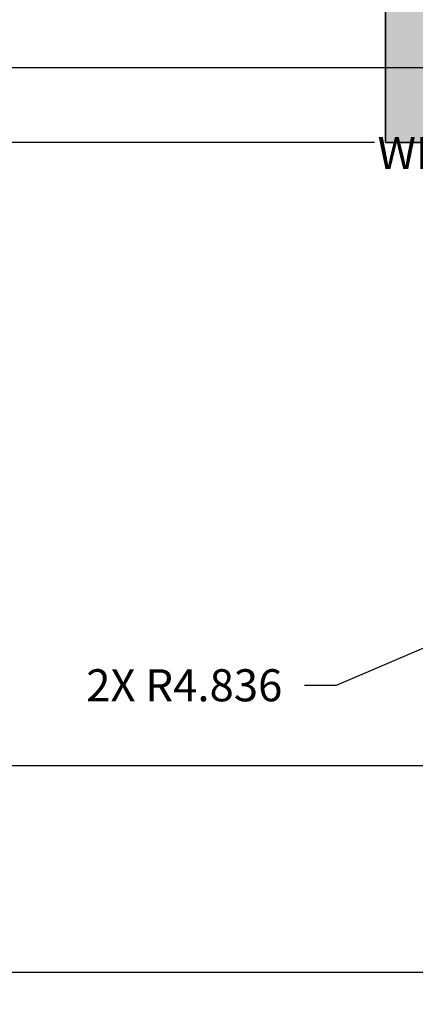
# Model space of a CAD drawing. Units: metres. Extents: x 4298.5 to 4325.2, y 2075 to 2095.8.
# Tile 2 of 35: x 4303.6 to 4305.8, y 2075 to 2080.5. Entities that reach past the tile are written whole.
import ezdxf

# ---------------------------------------------------------------- set-up
doc = ezdxf.new("R2010")
doc.units = ezdxf.units.M
for name, color, linetype, lineweight in [('A-ANNO-DIMS', 2, 'Continuous', 18), ('A-WALL', 7, 'Continuous', 35), ('A-WALL-PATT', 252, 'Continuous', 13)]:
    doc.layers.add(name, color=color, linetype=linetype, lineweight=lineweight)
doc.styles.get("Standard").update_dxf_attribs({"font": 'arial.ttf'})
doc.dimstyles.get("Standard").update_dxf_attribs({"dimtxt": 0.18, "dimasz": 0.18, "dimexe": 0.18, "dimexo": 0.0625, "dimgap": 0.09, "dimtad": 0, "dimtih": 1, "dimtoh": 1, "dimdec": 4, "dimzin": 0, "dimdsep": 46, "dimtxsty": 'Standard', "dimcen": 0.09, "dimadec": 0, "dimazin": 0, "dimtfac": 1, "dimtdec": 4, "dimtofl": 0, "dimtmove": 0, "dimatfit": 3, "dimfxl": 1, "dimtolj": 1, "dimtzin": 0, "dimarcsym": 0})

# ---------------------------------------------------------------- blocks, each defined once
blk = doc.blocks.new('*D23')
at = {"layer": 'A-ANNO-DIMS', "color": 0, "lineweight": -2, "transparency": 16777216}
for p, q in [((4308.1606, 2079.8556), (4308.1606, 2079.5881)), ((4309.1606, 2079.8556), (4309.1606, 2079.5881)), ((4308.1606, 2079.7681), (4307.9806, 2079.7681)), ((4308.9806, 2079.7681), (4308.3406, 2079.7681))]:
    blk.add_line(p, q, dxfattribs=at)
at = {"layer": 'A-ANNO-DIMS', "color": 0, "transparency": 16777216}
for points in [[(4308.3406, 2079.7981), (4308.3406, 2079.7381), (4308.1606, 2079.7681)], [(4308.9806, 2079.7981), (4308.9806, 2079.7381), (4309.1606, 2079.7681)]]:
    blk.add_solid(points, dxfattribs=at)
at = {"layer": 'Defpoints', "color": 0, "transparency": 16777216}
for p in [(4308.1606, 2079.9181), (4309.1606, 2079.9181), (4308.1606, 2079.7681)]:
    blk.add_point(p, dxfattribs=at)
at = {"layer": 'A-ANNO-DIMS', "color": 0, "transparency": 16777216, "insert": (4306.7086, 2079.7681), "char_height": 0.18, "attachment_point": 5}
blk.add_mtext('\\A1;WINDOW W1 1 TYP.', dxfattribs=at)
blk = doc.blocks.new('*D47')
at = {"layer": 'A-ANNO-DIMS', "color": 0, "lineweight": -2, "transparency": 16777216}
for p, q in [((4300.4306, 2084.4956), (4300.4306, 2074.9896)), ((4322.8106, 2084.4956), (4322.8106, 2074.9896)), ((4300.6106, 2075.1696), (4311.2252, 2075.1696)), ((4322.6306, 2075.1696), (4312.016, 2075.1696))]:
    blk.add_line(p, q, dxfattribs=at)
at = {"layer": 'A-ANNO-DIMS', "color": 0, "transparency": 16777216}
for points in [[(4300.6106, 2075.1996), (4300.6106, 2075.1396), (4300.4306, 2075.1696)], [(4322.6306, 2075.1996), (4322.6306, 2075.1396), (4322.8106, 2075.1696)]]:
    blk.add_solid(points, dxfattribs=at)
at = {"layer": 'Defpoints', "color": 0, "transparency": 16777216}
for p in [(4300.4306, 2084.5581), (4322.8106, 2084.5581), (4322.8106, 2075.1696)]:
    blk.add_point(p, dxfattribs=at)
at = {"layer": 'A-ANNO-DIMS', "color": 0, "transparency": 16777216, "insert": (4311.6206, 2075.1696), "char_height": 0.18, "attachment_point": 5}
blk.add_mtext('\\A1;22.38', dxfattribs=at)
blk = doc.blocks.new('*D51')
at = {"layer": 'A-ANNO-DIMS', "color": 0, "lineweight": -2, "transparency": 16777216}
for p, q in [((4305.5981, 2084.5581), (4299.0921, 2084.5581)), ((4299.2721, 2084.3781), (4299.2721, 2082.375)), ((4299.2721, 2080.0081), (4299.2721, 2082.0111)), ((4305.5981, 2079.8281), (4299.0921, 2079.8281))]:
    blk.add_line(p, q, dxfattribs=at)
at = {"layer": 'A-ANNO-DIMS', "color": 0, "transparency": 16777216}
for points in [[(4299.2421, 2084.3781), (4299.3021, 2084.3781), (4299.2721, 2084.5581)], [(4299.2421, 2080.0081), (4299.3021, 2080.0081), (4299.2721, 2079.8281)]]:
    blk.add_solid(points, dxfattribs=at)
at = {"layer": 'Defpoints', "color": 0, "transparency": 16777216}
for p in [(4305.6606, 2084.5581), (4299.2721, 2079.8281), (4305.6606, 2079.8281)]:
    blk.add_point(p, dxfattribs=at)
at = {"layer": 'A-ANNO-DIMS', "color": 0, "transparency": 16777216, "insert": (4299.2721, 2082.1931), "char_height": 0.18, "attachment_point": 5}
blk.add_mtext('\\A1;4.73', dxfattribs=at)
blk = doc.blocks.new('*D54')
at = {"layer": 'A-ANNO-DIMS', "color": 0, "lineweight": -2, "transparency": 16777216}
for p, q in [((4305.5981, 2079.8281), (4299.0921, 2079.8281)), ((4299.2721, 2079.6481), (4299.2721, 2078.26)), ((4299.2721, 2076.5081), (4299.2721, 2077.8961)), ((4309.0981, 2076.3281), (4299.0921, 2076.3281))]:
    blk.add_line(p, q, dxfattribs=at)
at = {"layer": 'A-ANNO-DIMS', "color": 0, "transparency": 16777216}
for points in [[(4299.2421, 2079.6481), (4299.3021, 2079.6481), (4299.2721, 2079.8281)], [(4299.2421, 2076.5081), (4299.3021, 2076.5081), (4299.2721, 2076.3281)]]:
    blk.add_solid(points, dxfattribs=at)
at = {"layer": 'Defpoints', "color": 0, "transparency": 16777216}
for p in [(4305.6606, 2079.8281), (4299.2721, 2076.3281), (4309.1606, 2076.3281)]:
    blk.add_point(p, dxfattribs=at)
at = {"layer": 'A-ANNO-DIMS', "color": 0, "transparency": 16777216, "insert": (4299.2721, 2078.0781), "char_height": 0.18, "attachment_point": 5}
blk.add_mtext('\\A1;3.5', dxfattribs=at)
blk = doc.blocks.new('*D64')
at = {"layer": 'A-ANNO-DIMS', "color": 0, "lineweight": -2, "transparency": 16777216}
for p, q in [((4312.1097, 2081.1221), (4299.0921, 2081.1221)), ((4299.2721, 2080.9421), (4299.2721, 2080.427)), ((4312.1097, 2080.247), (4299.0921, 2080.247)), ((4299.2721, 2080.247), (4299.2721, 2080.067)), ((4299.2721, 2080.067), (4299.0921, 2080.067))]:
    blk.add_line(p, q, dxfattribs=at)
at = {"layer": 'A-ANNO-DIMS', "color": 0, "transparency": 16777216}
for points in [[(4299.2421, 2080.9421), (4299.3021, 2080.9421), (4299.2721, 2081.1221)], [(4299.2421, 2080.427), (4299.3021, 2080.427), (4299.2721, 2080.247)]]:
    blk.add_solid(points, dxfattribs=at)
at = {"layer": 'Defpoints', "color": 0, "transparency": 16777216}
for p in [(4312.1722, 2081.1221), (4299.2721, 2080.247), (4312.1722, 2080.247)]:
    blk.add_point(p, dxfattribs=at)
at = {"layer": 'A-ANNO-DIMS', "color": 0, "transparency": 16777216, "insert": (4298.7681, 2080.067), "char_height": 0.18, "attachment_point": 5}
blk.add_mtext('\\A1;0.88', dxfattribs=at)
blk = doc.blocks.new('*D78')
at = {"layer": 'A-ANNO-DIMS', "color": 0, "lineweight": -2, "transparency": 16777216}
for p, q in [((4312.4969, 2079.7393), (4312.4969, 2079.9193)), ((4312.4069, 2079.8293), (4312.5869, 2079.8293)), ((4305.3847, 2076.7806), (4307.8863, 2077.853)), ((4305.2047, 2076.7806), (4305.3847, 2076.7806))]:
    blk.add_line(p, q, dxfattribs=at)
at = {"layer": 'A-ANNO-DIMS', "color": 0, "transparency": 16777216}
blk.add_solid([(4307.8745, 2077.8806), (4307.8981, 2077.8254), (4308.0518, 2077.9239)], dxfattribs=at)
at = {"layer": 'Defpoints', "color": 0, "transparency": 16777216}
for p in [(4312.4969, 2079.8293), (4308.0518, 2077.9239)]:
    blk.add_point(p, dxfattribs=at)
at = {"layer": 'A-ANNO-DIMS', "color": 0, "transparency": 16777216, "insert": (4304.53, 2076.7806), "char_height": 0.18, "attachment_point": 5}
blk.add_mtext('\\A1;2X R4.836', dxfattribs=at)

msp = doc.modelspace()

# ---------------------------------------------------------------- hatches: boundary and pattern name
at = {"layer": 'A-WALL-PATT'}
h = msp.add_hatch(color=256, dxfattribs=at)
h.dxf.hatch_style = 1
h.paths.add_polyline_path([(4308.7606, 2094.4781), (4308.1606, 2094.4781), (4307.4606, 2094.4781), (4307.4606, 2094.2481), (4308.2706, 2094.2481), (4308.2706, 2094.1281), (4308.3906, 2094.1281), (4308.3906, 2094.2481), (4308.7606, 2094.2481)])
h.paths.add_polyline_path([(4310.1206, 2094.4781), (4309.5206, 2094.4781), (4309.5206, 2094.2481), (4309.8906, 2094.2481), (4309.8906, 2092.2481), (4308.3906, 2092.2481), (4308.3906, 2093.4281), (4308.2706, 2093.4281), (4308.2706, 2092.0181), (4309.8906, 2092.0181), (4309.8906, 2087.0181), (4309.7706, 2087.0181), (4309.7706, 2086.7881), (4309.8906, 2086.7881), (4311.9406, 2086.7881), (4311.9406, 2087.0181), (4310.1206, 2087.0181), (4310.1206, 2089.0181), (4310.2406, 2089.0181), (4310.2406, 2089.1381), (4310.1206, 2089.1381), (4310.1206, 2092.0181), (4310.3078, 2092.0181), (4310.3078, 2092.2481), (4310.1206, 2092.2481)])
h.paths.add_polyline_path([(4311.7406, 2092.2481), (4311.0678, 2092.2481), (4311.0678, 2092.0181), (4311.7406, 2092.0181)], flags=17)
h.paths.add_polyline_path([(4313.1733, 2092.2481), (4312.5006, 2092.2481), (4312.5006, 2092.0181), (4313.1733, 2092.0181)])
h.paths.add_polyline_path([(4314.5378, 2092.2481), (4314.1206, 2092.2481), (4313.9333, 2092.2481), (4313.9333, 2092.0181), (4314.1206, 2092.0181), (4314.1206, 2087.0181), (4314.0006, 2087.0181), (4314.0006, 2086.7881), (4314.1206, 2086.7881), (4315.5718, 2086.7881), (4315.5718, 2087.0181), (4314.3506, 2087.0181), (4314.3506, 2092.0181), (4314.5378, 2092.0181)])
h.paths.add_polyline_path([(4315.9706, 2092.2481), (4315.2978, 2092.2481), (4315.2978, 2092.0181), (4315.9706, 2092.0181)])
h.paths.add_polyline_path([(4317.4033, 2092.2481), (4316.7306, 2092.2481), (4316.7306, 2092.0181), (4317.4033, 2092.0181)])
h.paths.add_polyline_path([(4318.9506, 2092.2481), (4318.3506, 2092.2481), (4318.1633, 2092.2481), (4318.1633, 2092.0181), (4318.3506, 2092.0181), (4318.3506, 2091.8981), (4318.5806, 2091.8981), (4318.5806, 2092.0181), (4318.9506, 2092.0181)])
h.paths.add_polyline_path([(4321.0106, 2092.2481), (4319.7106, 2092.2481), (4319.7106, 2092.0181), (4320.0806, 2092.0181), (4320.0806, 2090.0181), (4318.5806, 2090.0181), (4318.5806, 2091.1981), (4318.3506, 2091.1981), (4318.3506, 2090.0181), (4318.3506, 2087.0181), (4318.2306, 2087.0181), (4318.2306, 2086.7881), (4318.3506, 2086.7881), (4318.3506, 2086.3081), (4318.5806, 2086.3081), (4318.5806, 2089.7881), (4321.7806, 2089.7881), (4321.7806, 2090.0181), (4320.2006, 2090.0181), (4320.2006, 2092.0181), (4321.0106, 2092.0181)])
h.paths.add_polyline_path([(4322.8106, 2092.2481), (4321.7706, 2092.2481), (4321.7706, 2092.0181), (4322.5806, 2092.0181), (4322.5806, 2091.2831), (4322.8106, 2091.2831)])
h.paths.add_polyline_path([(4322.8106, 2090.5231), (4322.5806, 2090.5231), (4322.5806, 2089.7881), (4322.5806, 2089.5254), (4322.8106, 2089.5254), (4322.8106, 2090.0181)])
h.paths.add_polyline_path([(4322.8106, 2088.7654), (4322.5806, 2088.7654), (4322.5806, 2087.6681), (4322.8106, 2087.6681)])
h.paths.add_polyline_path([(4322.8106, 2086.9081), (4322.5806, 2086.9081), (4322.5806, 2085.8107), (4322.8106, 2085.8107)])
h.paths.add_polyline_path([(4322.8106, 2085.0507), (4322.5806, 2085.0507), (4322.5806, 2084.7881), (4318.5806, 2084.7881), (4318.5806, 2085.0581), (4318.5806, 2085.4081), (4318.3506, 2085.4081), (4318.3506, 2084.5581), (4318.3506, 2080.8581), (4318.4706, 2080.8581), (4318.4706, 2082.3281), (4319.2606, 2082.3281), (4319.2606, 2082.5581), (4318.5806, 2082.5581), (4318.5806, 2084.5581), (4320.0806, 2084.5581), (4320.0806, 2083.9381), (4320.3106, 2083.9381), (4320.3106, 2084.5581), (4322.8106, 2084.5581)])
h.paths.add_polyline_path([(4320.3106, 2083.1781), (4320.0806, 2083.1781), (4320.0806, 2082.5581), (4319.9606, 2082.5581), (4319.9606, 2082.3281), (4320.0806, 2082.3281), (4320.0806, 2081.5731), (4320.3106, 2081.5731)], flags=17)
h.paths.add_polyline_path([(4320.3106, 2080.8131), (4320.0806, 2080.8131), (4320.0806, 2080.0581), (4318.4286, 2080.0581), (4318.4286, 2079.8281), (4320.3106, 2079.8281)])
h.paths.add_polyline_path([(4317.3506, 2085.2881), (4316.5718, 2085.2881), (4316.5718, 2085.0581), (4317.3506, 2085.0581)])
h.paths.add_polyline_path([(4315.5718, 2085.2881), (4314.8434, 2085.2881), (4314.8434, 2085.0581), (4315.5718, 2085.0581)])
h.paths.add_polyline_path([(4313.8434, 2085.2881), (4312.9406, 2085.2881), (4312.9406, 2085.0581), (4313.8434, 2085.0581)])
h.paths.add_polyline_path([(4311.9406, 2085.2881), (4311.4406, 2085.2881), (4311.4406, 2085.0581), (4311.9406, 2085.0581)])
h.paths.add_polyline_path([(4317.3306, 2087.0181), (4316.5718, 2087.0181), (4316.5718, 2086.7881), (4317.3306, 2086.7881)])
h.paths.add_polyline_path([(4313.1006, 2089.1381), (4311.1406, 2089.1381), (4311.1406, 2089.0181), (4312.9806, 2089.0181), (4312.9806, 2087.0181), (4312.9406, 2087.0181), (4312.9406, 2086.7881), (4313.1006, 2086.7881), (4313.1006, 2087.0181)])
h.paths.add_polyline_path([(4307.5515, 2087.0181), (4305.8906, 2087.0181), (4305.8906, 2092.2481), (4305.8906, 2094.2481), (4306.7006, 2094.2481), (4306.7006, 2094.4781), (4305.6606, 2094.4781), (4305.6606, 2092.2481), (4305.2906, 2092.2481), (4305.2906, 2092.0181), (4305.6606, 2092.0181), (4305.6606, 2090.0181), (4304.1606, 2090.0181), (4304.1606, 2091.1981), (4304.0406, 2091.1981), (4304.0406, 2089.9081), (4301.5606, 2089.9081), (4301.5606, 2089.7881), (4304.0406, 2089.7881), (4305.6606, 2089.7881), (4305.6606, 2086.6381), (4305.8906, 2086.6381), (4305.8906, 2086.7881), (4307.5515, 2086.7881)])
h.paths.add_polyline_path([(4307.5515, 2085.2881), (4305.8906, 2085.2881), (4305.8906, 2085.4381), (4305.6606, 2085.4381), (4305.6606, 2084.7881), (4305.2906, 2084.7881), (4305.2906, 2084.5581), (4305.6606, 2084.5581), (4305.6606, 2084.02), (4305.8906, 2084.02), (4305.8906, 2084.5581), (4305.8906, 2085.0581), (4307.5515, 2085.0581)])
h.paths.add_polyline_path([(4310.2406, 2085.2881), (4308.5515, 2085.2881), (4308.5515, 2085.0581), (4310.2406, 2085.0581)])
h.paths.add_polyline_path([(4317.4286, 2080.0581), (4316.5718, 2080.0581), (4316.5718, 2079.8281), (4317.4286, 2079.8281)])
h.paths.add_polyline_path([(4315.5718, 2080.0581), (4314.8434, 2080.0581), (4314.8434, 2079.8281), (4315.5718, 2079.8281)])
h.paths.add_polyline_path([(4313.8434, 2080.0581), (4312.9406, 2080.0581), (4312.9406, 2079.8281), (4313.8434, 2079.8281)])
h.paths.add_polyline_path([(4311.9406, 2080.0581), (4311.4406, 2080.0581), (4311.4406, 2079.8281), (4311.9406, 2079.8281)])
h.paths.add_polyline_path([(4310.2406, 2080.0581), (4310.1206, 2080.0581), (4310.1206, 2084.0381), (4309.8906, 2084.0381), (4309.8906, 2080.0581), (4309.1606, 2080.0581), (4309.1606, 2079.8281), (4310.2406, 2079.8281)])
h.paths.add_polyline_path([(4308.1606, 2080.0581), (4307.5106, 2080.0581), (4307.5106, 2080.1781), (4307.3906, 2080.1781), (4307.3906, 2080.0581), (4305.8906, 2080.0581), (4305.8906, 2080.567), (4305.6606, 2080.567), (4305.6606, 2079.8281), (4308.1606, 2079.8281)])
h.paths.add_polyline_path([(4307.5106, 2081.9381), (4309.0906, 2081.9381), (4309.0906, 2082.0581), (4305.8906, 2082.0581), (4305.8906, 2083.26), (4305.6606, 2083.26), (4305.6606, 2081.327), (4305.8906, 2081.327), (4305.8906, 2081.9381), (4307.3906, 2081.9381), (4307.3906, 2080.8781), (4307.5106, 2080.8781)])
h.paths.add_polyline_path([(4304.5306, 2084.7881), (4302.7306, 2084.7881), (4302.7306, 2084.5581), (4304.5306, 2084.5581)])
h.paths.add_polyline_path([(4301.9706, 2084.7881), (4300.6606, 2084.7881), (4300.6606, 2085.0249), (4300.4306, 2085.0249), (4300.4306, 2084.5581), (4301.9706, 2084.5581)])
h.paths.add_polyline_path([(4300.6606, 2086.8843), (4300.4306, 2086.8843), (4300.4306, 2085.7849), (4300.6606, 2085.7849)])
h.paths.add_polyline_path([(4300.6606, 2089.1618), (4300.4306, 2089.1618), (4300.4306, 2087.6443), (4300.6606, 2087.6443)])
h.paths.add_polyline_path([(4300.6606, 2091.0212), (4300.4306, 2091.0212), (4300.4306, 2089.9218), (4300.6606, 2089.9218)])
h.paths.add_polyline_path([(4300.6606, 2092.0181), (4301.9706, 2092.0181), (4301.9706, 2092.2481), (4300.4306, 2092.2481), (4300.4306, 2091.7812), (4300.6606, 2091.7812)])
h.paths.add_polyline_path([(4304.5306, 2092.2481), (4302.7306, 2092.2481), (4302.7306, 2092.0181), (4304.0406, 2092.0181), (4304.0406, 2091.8981), (4304.1606, 2091.8981), (4304.1606, 2092.0181), (4304.5306, 2092.0181)], flags=17)

# ---------------------------------------------------------------- linework, layer by layer
at = {"layer": 'A-WALL'}
for p in [(4305.6606, 2084.5581), (4310.2406, 2079.8281)]:
    msp.add_line(p, (4305.6606, 2079.8281), dxfattribs=at)

# ---------------------------------------------------------------- dimensions: what is measured, and where the dimension line sits
at = {"layer": 'A-ANNO-DIMS'}
for base, p1, p2, override, picture, middle in [((4299.2721, 2079.8281), (4305.6606, 2084.5581), (4305.6606, 2079.8281), {"dimdec": 2, "dimlfac": 1, "dimrnd": 0, "dimzin": 0, "dimdsep": 46, "dimlunit": 2}, '*D51', (4299.2721, 2082.1931)), ((4299.2721, 2080.247), (4312.1722, 2081.1221), (4312.1722, 2080.247), {"dimdec": 2, "dimlfac": 1, "dimrnd": 0, "dimzin": 0, "dimdsep": 46, "dimlunit": 2}, '*D64', (4298.7681, 2080.067)), ((4299.2721, 2076.3281), (4305.6606, 2079.8281), (4309.1606, 2076.3281), {"dimdec": 1, "dimlfac": 1, "dimrnd": 0, "dimzin": 0, "dimdsep": 46, "dimlunit": 2}, '*D54', (4299.2721, 2078.0781))]:
    dim = msp.add_linear_dim(base=base, p1=p1, p2=p2, angle=90, dimstyle='Standard', override=override, dxfattribs=at)
    dim.commit()
    dim.dimension.update_dxf_attribs({"geometry": picture, "text_midpoint": middle})
dim = msp.add_linear_dim(base=(4322.8106, 2075.1696), p1=(4300.4306, 2084.5581), p2=(4322.8106, 2084.5581), dimstyle='Standard', override={"dimdec": 2, "dimlfac": 1, "dimrnd": 0, "dimzin": 0, "dimdsep": 46, "dimlunit": 2}, dxfattribs=at)
dim.commit()
dim.dimension.update_dxf_attribs({"geometry": '*D47', "text_midpoint": (4311.6206, 2075.1696)})
dim = msp.add_linear_dim(base=(4308.1606, 2079.7681), p1=(4309.1606, 2079.9181), p2=(4308.1606, 2079.9181), angle=180, text='WINDOW W1 <> TYP.', dimstyle='Standard', override={"dimdec": 0, "dimlfac": 1, "dimrnd": 0, "dimzin": 0, "dimdsep": 46, "dimlunit": 2}, dxfattribs=at)
dim.commit()
dim.dimension.update_dxf_attribs({"geometry": '*D23', "text_midpoint": (4306.7086, 2079.7681)})
dim = msp.add_radius_dim(center=(4312.4969, 2079.8293), mpoint=(4308.0518, 2077.9239), text='2X <>', dimstyle='Standard', override={"dimdec": 3, "dimlfac": 1, "dimrnd": 0, "dimzin": 0, "dimdsep": 46, "dimlunit": 2}, dxfattribs=at)
dim.commit()
dim.dimension.update_dxf_attribs({"geometry": '*D78', "text_midpoint": (4304.53, 2076.7806), "dimtype": 164})

doc.saveas('drawing.dxf')
